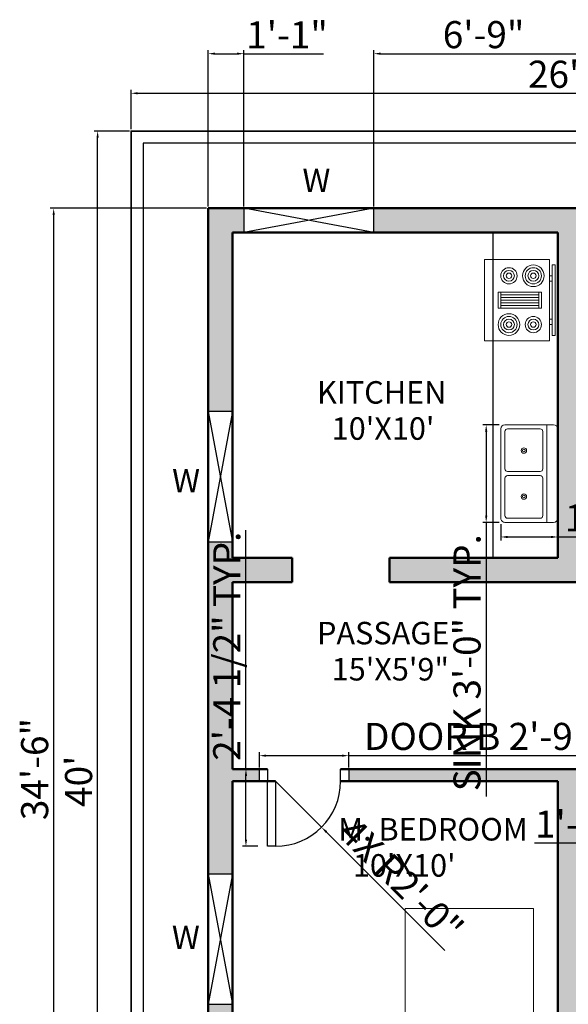
# Model space of a CAD drawing. Units: inches. Extents: x 2789 to 3623, y 2388 to 2993.
# Tile 4 of 5: x 3232 to 3435, y 2601 to 2964. Entities that reach past the tile are written whole.
import ezdxf

# ---------------------------------------------------------------- set-up
doc = ezdxf.new("R2010")
doc.units = ezdxf.units.IN
for name, color, linetype, lineweight in [('A-ANNO-DIMS', 2, 'Continuous', 18), ('A-ANNO-TEXT', 7, 'Continuous', 18), ('A-AREA-IDEN', 7, 'Continuous', 18), ('A-EQPM', 9, 'Continuous', 18), ('A-FLOR-CASE', 8, 'Continuous', 25), ('A-FLOR-FIXT', 9, 'Continuous', 18), ('A-FURN', 8, 'Continuous', 18), ('A-WALL', 7, 'Continuous', 50), ('A-WALL-PATT', 5, 'Continuous', 13), ('C-PROP', 7, 'Continuous', 35), ('d', 1, 'Continuous', 25), ('L-WALL', 7, 'Continuous', 25), ('w', 170, 'Continuous', 25)]:
    doc.layers.add(name, color=color, linetype=linetype, lineweight=lineweight)
doc.styles.get("Standard").update_dxf_attribs({"font": 'arial.ttf'})
doc.dimstyles.new('ISO-25', dxfattribs={"dimtxt": 10, "dimasz": 2.5, "dimexe": 1.25, "dimexo": 0.625, "dimtad": 1, "dimlunit": 4, "dimtxsty": 'Standard', "dimcen": 2.5, "dimadec": 0, "dimazin": 0, "dimtfac": 1, "dimtmove": 0, "dimatfit": 3, "dimfxl": 1, "dimarcsym": 0})

# ---------------------------------------------------------------- blocks, each defined once
blk = doc.blocks.new('Range-Oven - 30 in top')
for p, q in [((0, -3), (30, -3)), ((12, -6), (18, -6)), ((13, -20), (13, -6)), ((14, -6), (14, -20)), ((15, -20), (15, -6)), ((16, -6), (16, -20)), ((17, -20), (17, -6)), ((18, -20), (12, -20)), ((6, -24), (6, -25)), ((8, -25), (8, -24)), ((22, -25), (22, -24)), ((24, -24), (24, -25))]:
    blk.add_line(p, q)
for points in [[(0, -24), (0, 0), (30, 0), (30, -24)], [(12, -21), (12, -5), (18, -5), (18, -21)], [(2, -26), (2, -25), (28, -25), (28, -26)]]:
    blk.add_lwpolyline(points, close=True)
for centre, radius in [((6, -9), 4), ((6, -9), 3), ((6, -9), 2), ((24, -9), 3), ((24, -9), 2), ((6, -9), 1), ((24, -9), 1), ((24, -18), 4), ((6, -18), 3), ((6, -18), 2), ((6, -18), 1), ((24, -18), 3), ((24, -18), 2), ((24, -18), 1)]:
    blk.add_circle(centre, radius)
blk = doc.blocks.new('Sink-double - 36 in top')
for p, q in [((-18, -4), (18, -4)), ((-0.75, -18.5), (-0.75, -6.5)), ((0.75, -6.5), (0.75, -18.5))]:
    blk.add_line(p, q)
for points in [[(-16.5, 0), (16.5, 0)], [(-18, -19.5), (-18, -1.5)], [(18, -1.5), (18, -19.5)], [(-16.5, -18.5), (-16.5, -6.5)], [(-15.5, -5.5), (-1.75, -5.5)], [(1.75, -5.5), (15.5, -5.5)], [(16.5, -6.5), (16.5, -18.5)], [(16.5, -21), (-16.5, -21)], [(-1.75, -19.5), (-15.5, -19.5)], [(15.5, -19.5), (1.75, -19.5)]]:
    blk.add_lwpolyline(points)
for centre, radius in [((-8.5, -12.5), 1), ((-8.5, -12.5), 0.5), ((8.5, -12.5), 1), ((8.5, -12.5), 0.5)]:
    blk.add_circle(centre, radius)
for centre, radius, start, end in [((-16.5, -1.5), 1.5, 90, 180), ((16.5, -1.5), 1.5, 0, 90), ((-15.5, -6.5), 1, 90, 180), ((-1.75, -6.5), 1, 0, 90), ((1.75, -6.5), 1, 90, 180), ((15.5, -6.5), 1, 0, 90), ((-16.5, -19.5), 1.5, 180, 270), ((-15.5, -18.5), 1, 180, 270), ((-1.75, -18.5), 1, 270, 0), ((1.75, -18.5), 1, 180, 270), ((15.5, -18.5), 1, 270, 0), ((16.5, -19.5), 1.5, 270, 0)]:
    blk.add_arc(centre, radius, start, end)
blk = doc.blocks.new('Bed - Queen')
for p, q in [((0, -80.00003), (0, 0)), ((0, 0), (59.99999, 0)), ((59.99999, 0), (59.99999, -80.00003)), ((7.99999, -1.2), (28.79998, -1.2)), ((7.99999, -14.4), (7.99999, -1.2)), ((28.79998, -1.2), (28.79998, -14.4)), ((31.19999, -1.2), (51.99999, -1.2)), ((31.19999, -14.4), (31.19999, -1.2)), ((51.99999, -1.2), (51.99999, -16.4)), ((0, -14.4), (44.8, -14.4)), ((44.8, -16.8), (0, -16.8)), ((59.99999, -29.6), (44.8, -14.4)), ((44.8, -14.4), (44.8, -29.6)), ((51.99999, -16.4), (46.79936, -16.4)), ((44.8, -29.6), (59.99999, -29.6)), ((59.99999, -80.00003), (0, -80.00003))]:
    blk.add_line(p, q)
blk = doc.blocks.new('*D14')
at = {"layer": 'A-ANNO-DIMS', "color": 0, "lineweight": -2, "transparency": 16777216}
for p, q in [((3273.51, 2923.47), (3273.51, 2938.03)), ((3276.01, 2936.78), (3583.01, 2936.78)), ((3585.51, 2923.47), (3585.51, 2938.03))]:
    blk.add_line(p, q, dxfattribs=at)
at = {"layer": 'A-ANNO-DIMS', "color": 0, "transparency": 16777216}
for points in [[(3276.01, 2937.19), (3276.01, 2936.36), (3273.51, 2936.78)], [(3583.01, 2937.19), (3583.01, 2936.36), (3585.51, 2936.78)]]:
    blk.add_solid(points, dxfattribs=at)
at = {"layer": 'Defpoints', "color": 0, "transparency": 16777216}
for p in [(3585.51, 2936.78), (3273.51, 2922.84), (3585.51, 2922.84)]:
    blk.add_point(p, dxfattribs=at)
at = {"layer": 'A-ANNO-DIMS', "color": 0, "transparency": 16777216, "insert": (3429.51, 2942.51), "char_height": 10, "attachment_point": 5}
blk.add_mtext("26'", dxfattribs=at)
blk = doc.blocks.new('*D15')
at = {"layer": 'A-ANNO-DIMS', "color": 0, "lineweight": -2, "transparency": 16777216}
for p, q in [((3272.89, 2922.84), (3259.93, 2922.84)), ((3261.18, 2445.34), (3261.18, 2920.34)), ((3272.89, 2442.84), (3259.93, 2442.84))]:
    blk.add_line(p, q, dxfattribs=at)
at = {"layer": 'A-ANNO-DIMS', "color": 0, "transparency": 16777216}
for points in [[(3260.76, 2920.34), (3261.6, 2920.34), (3261.18, 2922.84)], [(3260.76, 2445.34), (3261.6, 2445.34), (3261.18, 2442.84)]]:
    blk.add_solid(points, dxfattribs=at)
at = {"layer": 'Defpoints', "color": 0, "transparency": 16777216}
for p in [(3261.18, 2922.84), (3273.51, 2922.84), (3273.51, 2442.84)]:
    blk.add_point(p, dxfattribs=at)
at = {"layer": 'A-ANNO-DIMS', "color": 0, "transparency": 16777216, "insert": (3255.45, 2682.84), "char_height": 10, "attachment_point": 5, "rotation": 90}
blk.add_mtext("40'", dxfattribs=at)
blk = doc.blocks.new('DOOR-24IN-JAMB-4_5IN')
for points in [[(-3, 0), (-6, 0), (-6, 4.5), (-3, 4.5)], [(27, 0), (24, 0), (24, 4.5), (27, 4.5)], [(0, -24), (-3, -24), (-3, 0), (0, 0)]]:
    blk.add_lwpolyline(points, close=True)
blk.add_arc((0, 0), 24, 270, 0)
blk = doc.blocks.new('WINDOW-48IN')
for p, q in [((48, 9), (0, 0)), ((48, 0), (0, 9))]:
    blk.add_line(p, q)
blk.add_lwpolyline([(0, 9), (0, 0), (48, 0), (48, 9)], close=True)
blk = doc.blocks.new('*D30')
at = {"layer": 'A-ANNO-DIMS', "color": 0, "lineweight": -2, "transparency": 16777216}
for p, q in [((3409.39, 2814.41), (3403.36, 2814.41)), ((3404.61, 2811.91), (3404.61, 2780.91)), ((3409.39, 2778.41), (3403.36, 2778.41)), ((3404.61, 2778.41), (3404.61, 2677.27))]:
    blk.add_line(p, q, dxfattribs=at)
at = {"layer": 'A-ANNO-DIMS', "color": 0, "transparency": 16777216}
for points in [[(3404.2, 2811.91), (3405.03, 2811.91), (3404.61, 2814.41)], [(3404.2, 2780.91), (3405.03, 2780.91), (3404.61, 2778.41)]]:
    blk.add_solid(points, dxfattribs=at)
at = {"layer": 'Defpoints', "color": 0, "transparency": 16777216}
for p in [(3410.01, 2814.41), (3404.61, 2778.41), (3410.01, 2778.41)]:
    blk.add_point(p, dxfattribs=at)
at = {"layer": 'A-ANNO-DIMS', "color": 0, "transparency": 16777216, "insert": (3398.82, 2726.59), "char_height": 10, "attachment_point": 5, "rotation": 90}
blk.add_mtext('SINK 3\'-0" TYP.', dxfattribs=at)
blk = doc.blocks.new('*D31')
at = {"layer": 'A-ANNO-DIMS', "color": 0, "lineweight": -2, "transparency": 16777216}
for p, q in [((3410.01, 2777.79), (3410.01, 2771.76)), ((3431.01, 2777.79), (3431.01, 2771.76)), ((3412.51, 2773.01), (3428.51, 2773.01)), ((3431.01, 2773.01), (3494.78, 2773.01))]:
    blk.add_line(p, q, dxfattribs=at)
at = {"layer": 'A-ANNO-DIMS', "color": 0, "transparency": 16777216}
for points in [[(3412.51, 2773.43), (3412.51, 2772.59), (3410.01, 2773.01)], [(3428.51, 2773.43), (3428.51, 2772.59), (3431.01, 2773.01)]]:
    blk.add_solid(points, dxfattribs=at)
at = {"layer": 'Defpoints', "color": 0, "transparency": 16777216}
for p in [(3410.01, 2778.41), (3431.01, 2778.41), (3431.01, 2773.01)]:
    blk.add_point(p, dxfattribs=at)
at = {"layer": 'A-ANNO-DIMS', "color": 0, "transparency": 16777216, "insert": (3464.15, 2778.74), "char_height": 10, "attachment_point": 5}
blk.add_mtext('1\'-9" TYP.', dxfattribs=at)
blk = doc.blocks.new('*D35')
at = {"layer": 'A-ANNO-DIMS', "color": 0, "lineweight": -2, "transparency": 16777216}
for p, q in [((3493.96, 2654.07), (3493.96, 2661.26)), ((3515.86, 2654.07), (3515.86, 2661.26)), ((3493.96, 2660.01), (3422.42, 2660.01)), ((3513.36, 2660.01), (3496.46, 2660.01))]:
    blk.add_line(p, q, dxfattribs=at)
at = {"layer": 'A-ANNO-DIMS', "color": 0, "transparency": 16777216}
for points in [[(3496.46, 2660.43), (3496.46, 2659.6), (3493.96, 2660.01)], [(3513.36, 2660.43), (3513.36, 2659.6), (3515.86, 2660.01)]]:
    blk.add_solid(points, dxfattribs=at)
at = {"layer": 'Defpoints', "color": 0, "transparency": 16777216}
for p in [(3493.96, 2660.01), (3493.96, 2653.44), (3515.86, 2653.44)]:
    blk.add_point(p, dxfattribs=at)
at = {"layer": 'A-ANNO-DIMS', "color": 0, "transparency": 16777216, "insert": (3456.94, 2665.74), "char_height": 10, "attachment_point": 5}
blk.add_mtext('1\'-10" TYP.', dxfattribs=at)
blk = doc.blocks.new('*D38')
at = {"layer": 'A-ANNO-DIMS', "color": 0, "lineweight": -2, "transparency": 16777216}
for p, q in [((3320.88, 2687.97), (3320.88, 2693.54)), ((3353.88, 2687.97), (3353.88, 2693.54)), ((3323.38, 2692.29), (3351.38, 2692.29)), ((3353.88, 2692.29), (3477.08, 2692.29))]:
    blk.add_line(p, q, dxfattribs=at)
at = {"layer": 'A-ANNO-DIMS', "color": 0, "transparency": 16777216}
for points in [[(3323.38, 2692.71), (3323.38, 2691.88), (3320.88, 2692.29)], [(3351.38, 2692.71), (3351.38, 2691.88), (3353.88, 2692.29)]]:
    blk.add_solid(points, dxfattribs=at)
at = {"layer": 'Defpoints', "color": 0, "transparency": 16777216}
for p in [(3353.88, 2692.29), (3320.88, 2687.34), (3353.88, 2687.34)]:
    blk.add_point(p, dxfattribs=at)
at = {"layer": 'A-ANNO-DIMS', "color": 0, "transparency": 16777216, "insert": (3416.73, 2698.09), "char_height": 10, "attachment_point": 5}
blk.add_mtext('DOOR B 2\'-9" TYP.', dxfattribs=at)
blk = doc.blocks.new('*D39')
at = {"layer": 'A-ANNO-DIMS', "color": 0, "lineweight": -2, "transparency": 16777216}
for p, q in [((3315.93, 2687.34), (3315.93, 2775.52)), ((3320.26, 2687.34), (3314.68, 2687.34)), ((3315.93, 2661.34), (3315.93, 2684.84)), ((3320.26, 2658.84), (3314.68, 2658.84))]:
    blk.add_line(p, q, dxfattribs=at)
at = {"layer": 'A-ANNO-DIMS', "color": 0, "transparency": 16777216}
for points in [[(3315.52, 2684.84), (3316.35, 2684.84), (3315.93, 2687.34)], [(3315.52, 2661.34), (3316.35, 2661.34), (3315.93, 2658.84)]]:
    blk.add_solid(points, dxfattribs=at)
at = {"layer": 'Defpoints', "color": 0, "transparency": 16777216}
for p in [(3315.93, 2687.34), (3320.88, 2687.34), (3320.88, 2658.84)]:
    blk.add_point(p, dxfattribs=at)
at = {"layer": 'A-ANNO-DIMS', "color": 0, "transparency": 16777216, "insert": (3310.14, 2732.68), "char_height": 10, "attachment_point": 5, "rotation": 90}
blk.add_mtext('2\'-4 1/2" TYP.', dxfattribs=at)
blk = doc.blocks.new('*D45')
at = {"layer": 'A-ANNO-DIMS', "color": 0, "lineweight": -2, "transparency": 16777216}
for p, q in [((3301.39, 2894.34), (3243.71, 2894.34)), ((3244.96, 2482.84), (3244.96, 2891.84)), ((3301.39, 2480.34), (3243.71, 2480.34))]:
    blk.add_line(p, q, dxfattribs=at)
at = {"layer": 'A-ANNO-DIMS', "color": 0, "transparency": 16777216}
for points in [[(3244.55, 2891.84), (3245.38, 2891.84), (3244.96, 2894.34)], [(3244.55, 2482.84), (3245.38, 2482.84), (3244.96, 2480.34)]]:
    blk.add_solid(points, dxfattribs=at)
at = {"layer": 'Defpoints', "color": 0, "transparency": 16777216}
for p in [(3244.96, 2894.34), (3302.01, 2894.34), (3302.01, 2480.34)]:
    blk.add_point(p, dxfattribs=at)
at = {"layer": 'A-ANNO-DIMS', "color": 0, "transparency": 16777216, "insert": (3239.23, 2687.34), "char_height": 10, "attachment_point": 5, "rotation": 90}
blk.add_mtext('34\'-6"', dxfattribs=at)
blk = doc.blocks.new('*D50')
at = {"layer": 'A-ANNO-DIMS', "color": 0, "lineweight": -2, "transparency": 16777216}
for p, q in [((3302.01, 2894.97), (3302.01, 2952.64)), ((3304.51, 2951.39), (3312.65, 2951.39)), ((3315.15, 2894.97), (3315.15, 2952.64)), ((3315.15, 2951.39), (3344.54, 2951.39))]:
    blk.add_line(p, q, dxfattribs=at)
at = {"layer": 'A-ANNO-DIMS', "color": 0, "transparency": 16777216}
for points in [[(3304.51, 2951.81), (3304.51, 2950.98), (3302.01, 2951.39)], [(3312.65, 2951.81), (3312.65, 2950.98), (3315.15, 2951.39)]]:
    blk.add_solid(points, dxfattribs=at)
at = {"layer": 'Defpoints', "color": 0, "transparency": 16777216}
for p in [(3315.15, 2951.39), (3302.01, 2894.34), (3315.15, 2894.34)]:
    blk.add_point(p, dxfattribs=at)
at = {"layer": 'A-ANNO-DIMS', "color": 0, "transparency": 16777216, "insert": (3331.1, 2957.04), "char_height": 10, "attachment_point": 5}
blk.add_mtext('1\'-1"', dxfattribs=at)
blk = doc.blocks.new('*D51')
at = {"layer": 'A-ANNO-DIMS', "color": 0, "lineweight": -2, "transparency": 16777216}
for p, q in [((3363.15, 2894.97), (3363.15, 2952.64)), ((3365.65, 2951.39), (3441.65, 2951.39)), ((3444.15, 2894.97), (3444.15, 2952.64))]:
    blk.add_line(p, q, dxfattribs=at)
at = {"layer": 'A-ANNO-DIMS', "color": 0, "transparency": 16777216}
for points in [[(3365.65, 2951.81), (3365.65, 2950.98), (3363.15, 2951.39)], [(3441.65, 2951.81), (3441.65, 2950.98), (3444.15, 2951.39)]]:
    blk.add_solid(points, dxfattribs=at)
at = {"layer": 'Defpoints', "color": 0, "transparency": 16777216}
for p in [(3444.15, 2951.39), (3363.15, 2894.34), (3444.15, 2894.34)]:
    blk.add_point(p, dxfattribs=at)
at = {"layer": 'A-ANNO-DIMS', "color": 0, "transparency": 16777216, "insert": (3403.65, 2957.12), "char_height": 10, "attachment_point": 5}
blk.add_mtext('6\'-9"', dxfattribs=at)
blk = doc.blocks.new('*D60')
at = {"layer": 'A-ANNO-DIMS', "color": 0, "lineweight": -2, "transparency": 16777216}
for p, q in [((3326.88, 2682.84), (3343.85, 2665.87)), ((3389.32, 2620.41), (3345.62, 2664.1))]:
    blk.add_line(p, q, dxfattribs=at)
at = {"layer": 'A-ANNO-DIMS', "color": 0, "transparency": 16777216}
blk.add_solid([(3345.92, 2664.4), (3345.33, 2663.81), (3343.85, 2665.87)], dxfattribs=at)
at = {"layer": 'Defpoints', "color": 0, "transparency": 16777216}
for p in [(3326.88, 2682.84), (3343.85, 2665.87)]:
    blk.add_point(p, dxfattribs=at)
at = {"layer": 'A-ANNO-DIMS', "color": 0, "transparency": 16777216, "insert": (3372.4, 2645.42), "char_height": 10, "attachment_point": 5, "rotation": 314.9998}
blk.add_mtext('4X R2\'-0"', dxfattribs=at)

msp = doc.modelspace()

# ---------------------------------------------------------------- hatches: boundary and pattern name
at = {"layer": 'A-WALL-PATT'}
h = msp.add_hatch(color=256, dxfattribs=at)
h.dxf.hatch_style = 1
h.paths.add_polyline_path([(3560.015, 2707.71), (3551.015, 2707.71), (3551.015, 2687.342), (3488.015, 2687.342), (3488.015, 2756.342), (3500.148, 2756.342), (3500.148, 2765.342), (3477.506, 2765.342), (3477.506, 2756.342), (3483.515, 2756.342), (3483.515, 2682.842), (3551.015, 2682.842), (3551.015, 2617.319), (3560.015, 2617.319)])
h.paths.add_polyline_path([(3560.015, 2817.229), (3551.015, 2817.229), (3551.015, 2812.239), (3551.015, 2765.342), (3533.148, 2765.342), (3533.148, 2756.342), (3551.015, 2756.342), (3551.015, 2731.71), (3560.015, 2731.71)])
h.paths.add_polyline_path([(3560.015, 2894.342), (3492.148, 2894.342), (3492.148, 2885.342), (3551.015, 2885.342), (3551.015, 2865.229), (3560.015, 2865.229)])
h.paths.add_polyline_path([(3444.148, 2894.342), (3363.151, 2894.342), (3363.151, 2885.342), (3431.015, 2885.342), (3431.015, 2765.342), (3368.943, 2765.342), (3368.943, 2756.342), (3444.506, 2756.342), (3444.506, 2765.342), (3440.015, 2765.342), (3440.015, 2885.342), (3444.148, 2885.342)])
h.paths.add_polyline_path([(3311.015, 2885.342), (3315.151, 2885.342), (3315.151, 2894.342), (3302.015, 2894.342), (3302.015, 2819.267), (3311.015, 2819.267)])
h.paths.add_polyline_path([(3311.015, 2756.342), (3332.943, 2756.342), (3332.943, 2765.342), (3311.015, 2765.342), (3311.015, 2771.267), (3302.015, 2771.267), (3302.015, 2648.516), (3311.015, 2648.516), (3311.015, 2682.842), (3320.883, 2682.842), (3320.883, 2687.342), (3311.015, 2687.342)])
h.paths.add_polyline_path([(3439.015, 2489.342), (3311.015, 2489.342), (3311.015, 2553.842), (3317.302, 2553.842), (3317.302, 2562.842), (3311.015, 2562.842), (3311.015, 2600.516), (3302.015, 2600.516), (3302.015, 2480.342), (3439.015, 2480.342)])
h.paths.add_polyline_path([(3447.515, 2562.842), (3440.015, 2562.842), (3440.015, 2687.342), (3353.883, 2687.342), (3353.883, 2682.842), (3431.015, 2682.842), (3431.015, 2562.842), (3365.302, 2562.842), (3365.302, 2553.842), (3447.515, 2553.842)])
h.paths.add_polyline_path([(3560.015, 2569.319), (3551.015, 2569.319), (3551.015, 2562.842), (3541.085, 2562.842), (3541.085, 2553.842), (3560.015, 2553.842)])
h.paths.add_polyline_path([(3439.015, 2523.092), (3359.015, 2523.092), (3359.015, 2520.092), (3439.015, 2520.092)], flags=17)
h.paths.add_polyline_path([(3341.726, 2503.274), (3341.726, 2543.14), (3329.011, 2543.14), (3329.011, 2503.274)], flags=25)
h.paths.add_polyline_path([(3328.42, 2497.829), (3328.42, 2542.718), (3315.535, 2542.718), (3315.535, 2497.829)], flags=25)
h.paths.add_polyline_path([(3476.819, 2492.441), (3529.584, 2492.441), (3529.584, 2505.156), (3476.819, 2505.156)], flags=9)
h.paths.add_polyline_path([(3482.427, 2505.748), (3529.241, 2505.748), (3529.241, 2518.633), (3482.427, 2518.633)], flags=9)
h.paths.add_polyline_path([(3491.312, 2778.023), (3533.511, 2778.023), (3533.511, 2790.738), (3491.312, 2790.738)], flags=9)
h.paths.add_polyline_path([(3467.584, 2791.33), (3549.839, 2791.33), (3549.839, 2804.214), (3467.584, 2804.214)], flags=9)
h.paths.add_polyline_path([(3489.974, 2712.567), (3519.954, 2712.567), (3519.954, 2720.13), (3489.974, 2720.13)], flags=25)
h.paths.add_polyline_path([(3493.529, 2720.481), (3522.128, 2720.481), (3522.128, 2728.14), (3493.529, 2728.14)], flags=25)
h.paths.add_polyline_path([(3443.312, 2609.496), (3485.511, 2609.496), (3485.511, 2622.211), (3443.312, 2622.211)], flags=9)
h.paths.add_polyline_path([(3444.938, 2623.016), (3478.097, 2623.016), (3478.097, 2635.468), (3444.938, 2635.468)], flags=9)
h.paths.add_polyline_path([(3353.282, 2645.374), (3395.481, 2645.374), (3395.481, 2658.089), (3353.282, 2658.089)], flags=9)
h.paths.add_polyline_path([(3347.837, 2658.68), (3428.155, 2658.68), (3428.155, 2671.565), (3347.837, 2671.565)], flags=9)
h.paths.add_polyline_path([(3345.461, 2717.778), (3391.776, 2717.778), (3391.776, 2730.493), (3345.461, 2730.493)], flags=9)
h.paths.add_polyline_path([(3340.017, 2731.086), (3399.739, 2731.086), (3399.739, 2743.962), (3340.017, 2743.962)], flags=9)
h.paths.add_polyline_path([(3345.461, 2806.621), (3387.66, 2806.621), (3387.66, 2819.336), (3345.461, 2819.336)], flags=9)
h.paths.add_polyline_path([(3340.017, 2819.929), (3398.431, 2819.929), (3398.431, 2832.806), (3340.017, 2832.806)], flags=9)

# ---------------------------------------------------------------- linework, layer by layer
at = {"layer": 'A-FLOR-CASE'}
msp.add_line((3407.015, 2885.342), (3407.015, 2765.342), dxfattribs=at)
at = {"layer": 'A-WALL'}
for p, q in [((3560.015, 2894.342), (3302.015, 2894.342)), ((3302.015, 2894.342), (3302.015, 2480.342)), ((3431.015, 2885.342), (3311.015, 2885.342)), ((3311.015, 2885.342), (3311.015, 2765.342)), ((3431.015, 2885.342), (3431.015, 2765.342)), ((3332.943, 2765.342), (3311.015, 2765.342)), ((3332.943, 2756.342), (3332.943, 2765.342)), ((3431.015, 2765.342), (3368.943, 2765.342)), ((3368.943, 2756.342), (3368.943, 2765.342)), ((3332.943, 2756.342), (3311.015, 2756.342)), ((3311.015, 2756.342), (3311.015, 2687.342)), ((3447.506, 2756.342), (3368.943, 2756.342)), ((3323.883, 2687.342), (3311.015, 2687.342)), ((3440.015, 2687.342), (3350.883, 2687.342)), ((3326.883, 2682.842), (3311.015, 2682.842)), ((3311.015, 2682.842), (3311.015, 2562.842)), ((3431.015, 2682.842), (3350.883, 2682.842)), ((3431.015, 2682.842), (3431.015, 2562.842))]:
    msp.add_line(p, q, dxfattribs=at)
at = {"layer": 'C-PROP'}
msp.add_lwpolyline([(3273.515, 2442.842), (3585.515, 2442.842), (3585.515, 2922.842), (3273.515, 2922.842)], close=True, dxfattribs=at)
at = {"layer": 'L-WALL'}
for p, q in [((3581.015, 2918.342), (3278.015, 2918.342)), ((3278.015, 2918.342), (3278.015, 2447.342))]:
    msp.add_line(p, q, dxfattribs=at)

# ---------------------------------------------------------------- block references
at = {"layer": 'A-EQPM', "rotation": 90}
msp.add_blockref('Range-Oven - 30 in top', (3404.015, 2845.404), dxfattribs=at)
at = {"layer": 'A-FLOR-FIXT', "rotation": 270}
msp.add_blockref('Sink-double - 36 in top', (3431.015, 2796.411), dxfattribs=at)
at = {"layer": 'A-FURN', "xscale": 0.7903362398625325, "yscale": 0.7903362398625325, "zscale": 0.7903362398625325, "rotation": 180}
msp.add_blockref('Bed - Queen', (3422.073, 2572.602), dxfattribs=at)
at = {"layer": 'd'}
msp.add_blockref('DOOR-24IN-JAMB-4_5IN', (3326.883, 2682.842), dxfattribs=at)
at = {"layer": 'w'}
msp.add_blockref('WINDOW-48IN', (3315.15, 2885.342), dxfattribs=at)
for p, rotation in [((3311.014, 2771.267), 90.0000000000013), ((3311.014, 2600.516), 90.00000000000095)]:
    msp.add_blockref('WINDOW-48IN', p, dxfattribs=dict(at, rotation=rotation))

# ---------------------------------------------------------------- texts
at = {"layer": 'A-ANNO-TEXT'}
for p in [(3336.79, 2900.34), (3288.684, 2789.502), (3288.596, 2620.935)]:
    msp.add_text('W', height=8.603, dxfattribs=at).set_placement(p)
at = {"layer": 'A-AREA-IDEN'}
for s, p in [('KITCHEN ', (3342.163, 2822.217)), ("10'X10'", (3347.58, 2808.882)), ('PASSAGE', (3342.163, 2733.374)), ('15\'X5\'9"', (3347.58, 2720.039)), ('M. BEDROOM', (3349.984, 2660.969)), ("10'X10'", (3355.401, 2647.635))]:
    msp.add_text(s, height=8.3011, dxfattribs=at).set_placement(p)

# ---------------------------------------------------------------- dimensions: what is measured, and where the dimension line sits
at = {"layer": 'A-ANNO-DIMS'}
for base, p1, p2, override, picture, middle in [((3315.151, 2951.392), (3302.015, 2894.342), (3315.151, 2894.342), {"dimdec": 1, "dimlfac": 1, "dimrnd": 0, "dimzin": 1, "dimdsep": 46, "dimlunit": 4, "dimfrac": 2}, '*D50', (3331.096, 2957.037)), ((3444.148, 2951.392), (3363.151, 2894.342), (3444.148, 2894.342), {"dimdec": 1, "dimlfac": 1, "dimrnd": 0, "dimzin": 1, "dimdsep": 46, "dimlunit": 4, "dimfrac": 2}, '*D51', (3403.649, 2957.122)), ((3585.515, 2936.777), (3273.515, 2922.842), (3585.515, 2922.842), {"dimclrd": 0, "dimclre": 0, "dimclrt": 0}, '*D14', (3429.515, 2942.508))]:
    dim = msp.add_linear_dim(base=base, p1=p1, p2=p2, dimstyle='ISO-25', override=override, dxfattribs=at)
    dim.commit()
    dim.dimension.update_dxf_attribs({"geometry": picture, "text_midpoint": middle})
for base, p1, p2, override, picture, middle in [((3261.179, 2922.842), (3273.515, 2442.842), (3273.515, 2922.842), {"dimclrd": 0, "dimclre": 0, "dimclrt": 0}, '*D15', (3255.448, 2682.842)), ((3244.965, 2894.342), (3302.015, 2480.342), (3302.015, 2894.342), {"dimdec": 1, "dimlfac": 1, "dimrnd": 0, "dimzin": 1, "dimdsep": 46, "dimlunit": 4, "dimfrac": 2}, '*D45', (3239.23, 2687.342))]:
    dim = msp.add_linear_dim(base=base, p1=p1, p2=p2, angle=90, dimstyle='ISO-25', override=override, dxfattribs=at)
    dim.commit()
    dim.dimension.update_dxf_attribs({"geometry": picture, "text_midpoint": middle})
for base, p1, p2, angle, text, picture, middle in [((3404.615, 2778.411), (3410.015, 2814.411), (3410.015, 2778.411), 270, 'SINK <> TYP.', '*D30', (3398.816, 2726.588)), ((3315.933, 2687.342), (3320.883, 2658.842), (3320.883, 2687.342), 90, '<> TYP.', '*D39', (3310.138, 2732.68)), ((3493.955, 2660.014), (3515.863, 2653.442), (3493.955, 2653.442), 180, '<> TYP.', '*D35', (3456.939, 2665.745))]:
    dim = msp.add_linear_dim(base=base, p1=p1, p2=p2, angle=angle, text=text, dimstyle='ISO-25', override={"dimdec": 1, "dimlfac": 1, "dimrnd": 0, "dimzin": 1, "dimdsep": 46, "dimlunit": 4, "dimfrac": 2}, dxfattribs=at)
    dim.commit()
    dim.dimension.update_dxf_attribs({"geometry": picture, "text_midpoint": middle})
for base, p1, p2, text, picture, middle in [((3431.015, 2773.011), (3410.015, 2778.411), (3431.015, 2778.411), '<> TYP.', '*D31', (3464.146, 2778.741)), ((3353.883, 2692.292), (3320.883, 2687.342), (3353.883, 2687.342), 'DOOR B <> TYP.', '*D38', (3416.732, 2698.091))]:
    dim = msp.add_linear_dim(base=base, p1=p1, p2=p2, text=text, dimstyle='ISO-25', override={"dimdec": 1, "dimlfac": 1, "dimrnd": 0, "dimzin": 1, "dimdsep": 46, "dimlunit": 4, "dimfrac": 2}, dxfattribs=at)
    dim.commit()
    dim.dimension.update_dxf_attribs({"geometry": picture, "text_midpoint": middle})
dim = msp.add_radius_dim(center=(3326.883, 2682.842), mpoint=(3343.854, 2665.871), text='4X <>', dimstyle='ISO-25', override={"dimdec": 1, "dimlfac": 1, "dimrnd": 0, "dimzin": 1, "dimdsep": 46, "dimlunit": 4, "dimfrac": 2}, dxfattribs=at)
dim.commit()
dim.dimension.update_dxf_attribs({"geometry": '*D60', "text_midpoint": (3372.405, 2645.425)})

doc.saveas('drawing.dxf')
